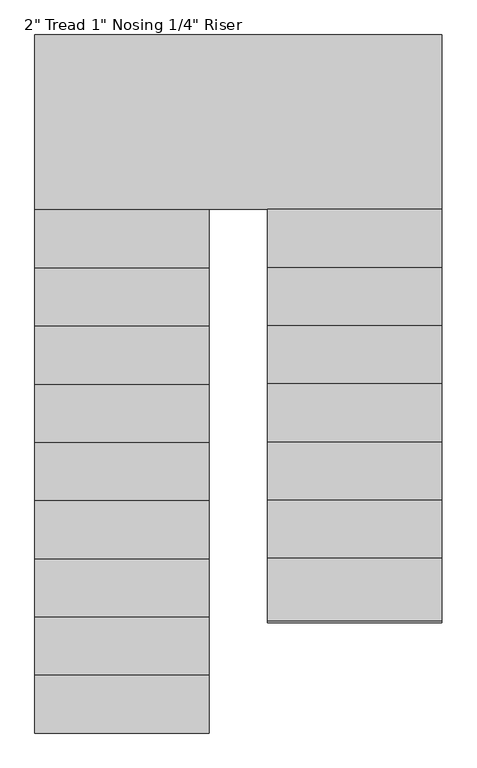
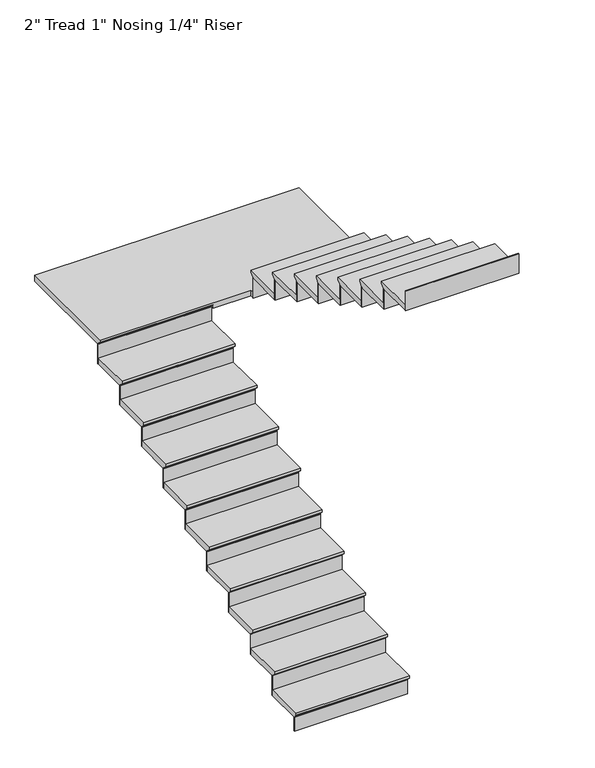
"""IFC4 building model written with IfcOpenShell, lengths in millimetres: stair flight geometry."""

from ifc_helpers import new_model, si_unit, origin, place, context, project, spatial, faceted_brep, source, transform, mapped, element, save


def stair_flight_2b6aeb10(model_context):
    return source(origin(), model_context, "Body", "Brep", [
        faceted_brep([(-77.7175798, -5516.2061634, 455.0833333), (-77.7175798, -5516.2061634, 474.1333333), (-992.1175798, -5516.2061634, 474.1333333), (-992.1175798, -5516.2061634, 455.0833333), (-77.7175798, -5490.8061634, 429.6833333), (-992.1175798, -5490.8061634, 429.6833333), (-77.7175798, -5186.0061634, 474.1333333), (-992.1175798, -5186.0061634, 474.1333333), (-992.1175798, -5490.8061634, 423.3333333), (-992.1175798, -5186.0061634, 423.3333333), (-77.7175798, -5186.0061634, 423.3333333), (-77.7175798, -5490.8061634, 423.3333333)], [[[0, 1, 2, 3]], [[4, 0, 3, 5]], [[2, 1, 6, 7]], [[8, 9, 10, 11]], [[2, 7, 9, 8, 5, 3]], [[8, 11, 4, 5]], [[6, 1, 0, 4, 11, 10]], [[7, 6, 10, 9]]]),
        faceted_brep([(-77.7175798, -5490.8061634, 423.3333333), (-77.7175798, -5490.8061634, 304.8), (-77.7175798, -5484.4561634, 304.8), (-77.7175798, -5484.4561634, 423.3333333), (-992.1175798, -5490.8061634, 423.3333333), (-992.1175798, -5484.4561634, 423.3333333), (-992.1175798, -5484.4561634, 304.8), (-992.1175798, -5490.8061634, 304.8)], [[[0, 1, 2, 3]], [[4, 5, 6, 7]], [[1, 0, 4, 7]], [[2, 1, 7, 6]], [[3, 2, 6, 5]], [[0, 3, 5, 4]]]),
        faceted_brep([(-77.7175798, -5186.0061634, 592.6666667), (-77.7175798, -5186.0061634, 423.3333333), (-77.7175798, -5179.6561634, 423.3333333), (-77.7175798, -5179.6561634, 592.6666667), (-992.1175798, -5186.0061634, 592.6666667), (-992.1175798, -5179.6561634, 592.6666667), (-992.1175798, -5179.6561634, 423.3333333), (-992.1175798, -5186.0061634, 423.3333333)], [[[0, 1, 2, 3]], [[4, 5, 6, 7]], [[1, 0, 4, 7]], [[2, 1, 7, 6]], [[3, 2, 6, 5]], [[0, 3, 5, 4]]]),
        faceted_brep([(-992.1175798, -5211.4061634, 643.4666667), (-77.7175798, -5211.4061634, 643.4666667), (-77.7175798, -4881.2061634, 643.4666667), (-992.1175798, -4881.2061634, 643.4666667), (-992.1175798, -5186.0061634, 592.6666667), (-992.1175798, -4881.2061634, 592.6666667), (-77.7175798, -4881.2061634, 592.6666667), (-77.7175798, -5186.0061634, 592.6666667), (-992.1175798, -5186.0061634, 599.0166667), (-992.1175798, -5211.4061634, 624.4166667), (-77.7175798, -5186.0061634, 599.0166667), (-77.7175798, -5211.4061634, 624.4166667)], [[[0, 1, 2, 3]], [[4, 5, 6, 7]], [[0, 3, 5, 4, 8, 9]], [[4, 7, 10, 8]], [[2, 1, 11, 10, 7, 6]], [[3, 2, 6, 5]], [[11, 1, 0, 9]], [[10, 11, 9, 8]]]),
        faceted_brep([(-77.7175798, -4881.2061634, 762.0), (-77.7175798, -4881.2061634, 592.6666667), (-77.7175798, -4874.8561634, 592.6666667), (-77.7175798, -4874.8561634, 762.0), (-992.1175798, -4881.2061634, 762.0), (-992.1175798, -4874.8561634, 762.0), (-992.1175798, -4874.8561634, 592.6666667), (-992.1175798, -4881.2061634, 592.6666667)], [[[0, 1, 2, 3]], [[4, 5, 6, 7]], [[1, 0, 4, 7]], [[2, 1, 7, 6]], [[3, 2, 6, 5]], [[0, 3, 5, 4]]]),
        faceted_brep([(-992.1175798, -4906.6061634, 812.8), (-77.7175798, -4906.6061634, 812.8), (-77.7175798, -4576.4061634, 812.8), (-992.1175798, -4576.4061634, 812.8), (-992.1175798, -4881.2061634, 762.0), (-992.1175798, -4576.4061634, 762.0), (-77.7175798, -4576.4061634, 762.0), (-77.7175798, -4881.2061634, 762.0), (-992.1175798, -4881.2061634, 768.35), (-992.1175798, -4906.6061634, 793.75), (-77.7175798, -4881.2061634, 768.35), (-77.7175798, -4906.6061634, 793.75)], [[[0, 1, 2, 3]], [[4, 5, 6, 7]], [[0, 3, 5, 4, 8, 9]], [[4, 7, 10, 8]], [[2, 1, 11, 10, 7, 6]], [[3, 2, 6, 5]], [[11, 1, 0, 9]], [[10, 11, 9, 8]]]),
        faceted_brep([(-77.7175798, -4576.4061634, 931.3333333), (-77.7175798, -4576.4061634, 762.0), (-77.7175798, -4570.0561634, 762.0), (-77.7175798, -4570.0561634, 931.3333333), (-992.1175798, -4576.4061634, 931.3333333), (-992.1175798, -4570.0561634, 931.3333333), (-992.1175798, -4570.0561634, 762.0), (-992.1175798, -4576.4061634, 762.0)], [[[0, 1, 2, 3]], [[4, 5, 6, 7]], [[1, 0, 4, 7]], [[2, 1, 7, 6]], [[3, 2, 6, 5]], [[0, 3, 5, 4]]]),
        faceted_brep([(-992.1175798, -4601.8061634, 982.1333333), (-77.7175798, -4601.8061634, 982.1333333), (-77.7175798, -4271.6061634, 982.1333333), (-992.1175798, -4271.6061634, 982.1333333), (-992.1175798, -4576.4061634, 931.3333333), (-992.1175798, -4271.6061634, 931.3333333), (-77.7175798, -4271.6061634, 931.3333333), (-77.7175798, -4576.4061634, 931.3333333), (-992.1175798, -4576.4061634, 937.6833333), (-992.1175798, -4601.8061634, 963.0833333), (-77.7175798, -4576.4061634, 937.6833333), (-77.7175798, -4601.8061634, 963.0833333)], [[[0, 1, 2, 3]], [[4, 5, 6, 7]], [[0, 3, 5, 4, 8, 9]], [[4, 7, 10, 8]], [[2, 1, 11, 10, 7, 6]], [[3, 2, 6, 5]], [[11, 1, 0, 9]], [[10, 11, 9, 8]]]),
        faceted_brep([(-77.7175798, -4271.6061634, 1100.6666667), (-77.7175798, -4271.6061634, 931.3333333), (-77.7175798, -4265.2561634, 931.3333333), (-77.7175798, -4265.2561634, 1100.6666667), (-992.1175798, -4271.6061634, 1100.6666667), (-992.1175798, -4265.2561634, 1100.6666667), (-992.1175798, -4265.2561634, 931.3333333), (-992.1175798, -4271.6061634, 931.3333333)], [[[0, 1, 2, 3]], [[4, 5, 6, 7]], [[1, 0, 4, 7]], [[2, 1, 7, 6]], [[3, 2, 6, 5]], [[0, 3, 5, 4]]]),
        faceted_brep([(-992.1175798, -4297.0061634, 1151.4666667), (-77.7175798, -4297.0061634, 1151.4666667), (-77.7175798, -3966.8061634, 1151.4666667), (-992.1175798, -3966.8061634, 1151.4666667), (-992.1175798, -4271.6061634, 1100.6666667), (-992.1175798, -3966.8061634, 1100.6666667), (-77.7175798, -3966.8061634, 1100.6666667), (-77.7175798, -4271.6061634, 1100.6666667), (-992.1175798, -4271.6061634, 1107.0166667), (-992.1175798, -4297.0061634, 1132.4166667), (-77.7175798, -4271.6061634, 1107.0166667), (-77.7175798, -4297.0061634, 1132.4166667)], [[[0, 1, 2, 3]], [[4, 5, 6, 7]], [[0, 3, 5, 4, 8, 9]], [[4, 7, 10, 8]], [[2, 1, 11, 10, 7, 6]], [[3, 2, 6, 5]], [[11, 1, 0, 9]], [[10, 11, 9, 8]]]),
        faceted_brep([(-77.7175798, -3966.8061634, 1270.0), (-77.7175798, -3966.8061634, 1100.6666667), (-77.7175798, -3960.4561634, 1100.6666667), (-77.7175798, -3960.4561634, 1270.0), (-992.1175798, -3966.8061634, 1270.0), (-992.1175798, -3960.4561634, 1270.0), (-992.1175798, -3960.4561634, 1100.6666667), (-992.1175798, -3966.8061634, 1100.6666667)], [[[0, 1, 2, 3]], [[4, 5, 6, 7]], [[1, 0, 4, 7]], [[2, 1, 7, 6]], [[3, 2, 6, 5]], [[0, 3, 5, 4]]]),
        faceted_brep([(-992.1175798, -3992.2061634, 1320.8), (-77.7175798, -3992.2061634, 1320.8), (-77.7175798, -3662.0061634, 1320.8), (-992.1175798, -3662.0061634, 1320.8), (-992.1175798, -3966.8061634, 1270.0), (-992.1175798, -3662.0061634, 1270.0), (-77.7175798, -3662.0061634, 1270.0), (-77.7175798, -3966.8061634, 1270.0), (-992.1175798, -3966.8061634, 1276.35), (-992.1175798, -3992.2061634, 1301.75), (-77.7175798, -3966.8061634, 1276.35), (-77.7175798, -3992.2061634, 1301.75)], [[[0, 1, 2, 3]], [[4, 5, 6, 7]], [[0, 3, 5, 4, 8, 9]], [[4, 7, 10, 8]], [[2, 1, 11, 10, 7, 6]], [[3, 2, 6, 5]], [[11, 1, 0, 9]], [[10, 11, 9, 8]]]),
        faceted_brep([(-77.7175798, -3662.0061634, 1439.3333333), (-77.7175798, -3662.0061634, 1270.0), (-77.7175798, -3655.6561634, 1270.0), (-77.7175798, -3655.6561634, 1439.3333333), (-992.1175798, -3662.0061634, 1439.3333333), (-992.1175798, -3655.6561634, 1439.3333333), (-992.1175798, -3655.6561634, 1270.0), (-992.1175798, -3662.0061634, 1270.0)], [[[0, 1, 2, 3]], [[4, 5, 6, 7]], [[1, 0, 4, 7]], [[2, 1, 7, 6]], [[3, 2, 6, 5]], [[0, 3, 5, 4]]]),
        faceted_brep([(-992.1175798, -3687.4061634, 1490.1333333), (-77.7175798, -3687.4061634, 1490.1333333), (-77.7175798, -3357.2061634, 1490.1333333), (-992.1175798, -3357.2061634, 1490.1333333), (-992.1175798, -3662.0061634, 1439.3333333), (-992.1175798, -3357.2061634, 1439.3333333), (-77.7175798, -3357.2061634, 1439.3333333), (-77.7175798, -3662.0061634, 1439.3333333), (-992.1175798, -3662.0061634, 1445.6833333), (-992.1175798, -3687.4061634, 1471.0833333), (-77.7175798, -3662.0061634, 1445.6833333), (-77.7175798, -3687.4061634, 1471.0833333)], [[[0, 1, 2, 3]], [[4, 5, 6, 7]], [[0, 3, 5, 4, 8, 9]], [[4, 7, 10, 8]], [[2, 1, 11, 10, 7, 6]], [[3, 2, 6, 5]], [[11, 1, 0, 9]], [[10, 11, 9, 8]]]),
        faceted_brep([(-77.7175798, -3357.2061634, 1608.6666667), (-77.7175798, -3357.2061634, 1439.3333333), (-77.7175798, -3350.8561634, 1439.3333333), (-77.7175798, -3350.8561634, 1608.6666667), (-992.1175798, -3357.2061634, 1608.6666667), (-992.1175798, -3350.8561634, 1608.6666667), (-992.1175798, -3350.8561634, 1439.3333333), (-992.1175798, -3357.2061634, 1439.3333333)], [[[0, 1, 2, 3]], [[4, 5, 6, 7]], [[1, 0, 4, 7]], [[2, 1, 7, 6]], [[3, 2, 6, 5]], [[0, 3, 5, 4]]]),
        faceted_brep([(-992.1175798, -3382.6061634, 1659.4666667), (-77.7175798, -3382.6061634, 1659.4666667), (-77.7175798, -3052.4061634, 1659.4666667), (-992.1175798, -3052.4061634, 1659.4666667), (-992.1175798, -3357.2061634, 1608.6666667), (-992.1175798, -3052.4061634, 1608.6666667), (-77.7175798, -3052.4061634, 1608.6666667), (-77.7175798, -3357.2061634, 1608.6666667), (-992.1175798, -3357.2061634, 1615.0166667), (-992.1175798, -3382.6061634, 1640.4166667), (-77.7175798, -3357.2061634, 1615.0166667), (-77.7175798, -3382.6061634, 1640.4166667)], [[[0, 1, 2, 3]], [[4, 5, 6, 7]], [[0, 3, 5, 4, 8, 9]], [[4, 7, 10, 8]], [[2, 1, 11, 10, 7, 6]], [[3, 2, 6, 5]], [[11, 1, 0, 9]], [[10, 11, 9, 8]]]),
        faceted_brep([(-77.7175798, -3052.4061634, 1778.0), (-77.7175798, -3052.4061634, 1608.6666667), (-77.7175798, -3046.0561634, 1608.6666667), (-77.7175798, -3046.0561634, 1778.0), (-992.1175798, -3052.4061634, 1778.0), (-992.1175798, -3046.0561634, 1778.0), (-992.1175798, -3046.0561634, 1608.6666667), (-992.1175798, -3052.4061634, 1608.6666667)], [[[0, 1, 2, 3]], [[4, 5, 6, 7]], [[1, 0, 4, 7]], [[2, 1, 7, 6]], [[3, 2, 6, 5]], [[0, 3, 5, 4]]]),
        faceted_brep([(-992.1175798, -3077.8061634, 1828.8), (-77.7175798, -3077.8061634, 1828.8), (-77.7175798, -2747.6061634, 1828.8), (-992.1175798, -2747.6061634, 1828.8), (-992.1175798, -3052.4061634, 1778.0), (-992.1175798, -2747.6061634, 1778.0), (-77.7175798, -2747.6061634, 1778.0), (-77.7175798, -3052.4061634, 1778.0), (-992.1175798, -3052.4061634, 1784.35), (-992.1175798, -3077.8061634, 1809.75), (-77.7175798, -3052.4061634, 1784.35), (-77.7175798, -3077.8061634, 1809.75)], [[[0, 1, 2, 3]], [[4, 5, 6, 7]], [[0, 3, 5, 4, 8, 9]], [[4, 7, 10, 8]], [[2, 1, 11, 10, 7, 6]], [[3, 2, 6, 5]], [[11, 1, 0, 9]], [[10, 11, 9, 8]]]),
        faceted_brep([(-77.7175798, -2747.6061634, 1947.3333333), (-77.7175798, -2747.6061634, 1778.0), (-77.7175798, -2741.2561634, 1778.0), (-77.7175798, -2741.2561634, 1947.3333333), (-992.1175798, -2747.6061634, 1947.3333333), (-992.1175798, -2741.2561634, 1947.3333333), (-992.1175798, -2741.2561634, 1778.0), (-992.1175798, -2747.6061634, 1778.0)], [[[0, 1, 2, 3]], [[4, 5, 6, 7]], [[1, 0, 4, 7]], [[2, 1, 7, 6]], [[3, 2, 6, 5]], [[0, 3, 5, 4]]]),
        faceted_brep([(1141.4824202, -2798.4061634, 1998.1333333), (1141.4824202, -1858.6061634, 1998.1333333), (-992.1175798, -1858.6061634, 1998.1333333), (-992.1175798, -2773.0061634, 1998.1333333), (227.0824202, -2773.0061634, 1998.1333333), (227.0824202, -2798.4061634, 1998.1333333), (1141.4824202, -1858.6061634, 1947.3333333), (1141.4824202, -2798.4061634, 1947.3333333), (227.0824202, -2798.4061634, 1947.3333333), (227.0824202, -2773.0061634, 1947.3333333), (-77.7175798, -2773.0061634, 1947.3333333), (-77.7175798, -2747.6061634, 1947.3333333), (-992.1175798, -2747.6061634, 1947.3333333), (-992.1175798, -1858.6061634, 1947.3333333), (-992.1175798, -2747.6061634, 1953.6833333), (-992.1175798, -2773.0061634, 1979.0833333), (-77.7175798, -2747.6061634, 1953.6833333), (-77.7175798, -2773.0061634, 1979.0833333)], [[[0, 1, 2, 3, 4, 5]], [[6, 7, 8, 9, 10, 11, 12, 13]], [[1, 0, 7, 6]], [[2, 1, 6, 13]], [[3, 2, 13, 12, 14, 15]], [[12, 11, 16, 14]], [[11, 10, 17, 16]], [[4, 3, 15, 17, 10, 9]], [[5, 4, 9, 8]], [[0, 5, 8, 7]], [[15, 14, 16, 17]]]),
        faceted_brep([(227.0824202, -2798.4061634, 2116.6666667), (227.0824202, -2798.4061634, 1947.3333333), (227.0824202, -2804.7561634, 1947.3333333), (227.0824202, -2804.7561634, 2116.6666667), (1141.4824202, -2798.4061634, 2116.6666667), (1141.4824202, -2804.7561634, 2116.6666667), (1141.4824202, -2804.7561634, 1947.3333333), (1141.4824202, -2798.4061634, 1947.3333333)], [[[0, 1, 2, 3]], [[4, 5, 6, 7]], [[1, 0, 4, 7]], [[2, 1, 7, 6]], [[3, 2, 6, 5]], [[0, 3, 5, 4]]]),
        faceted_brep([(1141.4824202, -2773.0061634, 2167.4666667), (227.0824202, -2773.0061634, 2167.4666667), (227.0824202, -3103.2061634, 2167.4666667), (1141.4824202, -3103.2061634, 2167.4666667), (1141.4824202, -2798.4061634, 2116.6666667), (1141.4824202, -3103.2061634, 2116.6666667), (227.0824202, -3103.2061634, 2116.6666667), (227.0824202, -2798.4061634, 2116.6666667), (1141.4824202, -2798.4061634, 2123.0166667), (1141.4824202, -2773.0061634, 2148.4166667), (227.0824202, -2798.4061634, 2123.0166667), (227.0824202, -2773.0061634, 2148.4166667)], [[[0, 1, 2, 3]], [[4, 5, 6, 7]], [[0, 3, 5, 4, 8, 9]], [[4, 7, 10, 8]], [[2, 1, 11, 10, 7, 6]], [[3, 2, 6, 5]], [[11, 1, 0, 9]], [[10, 11, 9, 8]]]),
        faceted_brep([(227.0824202, -3103.2061634, 2286.0), (227.0824202, -3103.2061634, 2116.6666667), (227.0824202, -3109.5561634, 2116.6666667), (227.0824202, -3109.5561634, 2286.0), (1141.4824202, -3103.2061634, 2286.0), (1141.4824202, -3109.5561634, 2286.0), (1141.4824202, -3109.5561634, 2116.6666667), (1141.4824202, -3103.2061634, 2116.6666667)], [[[0, 1, 2, 3]], [[4, 5, 6, 7]], [[1, 0, 4, 7]], [[2, 1, 7, 6]], [[3, 2, 6, 5]], [[0, 3, 5, 4]]]),
        faceted_brep([(1141.4824202, -3077.8061634, 2336.8), (227.0824202, -3077.8061634, 2336.8), (227.0824202, -3408.0061634, 2336.8), (1141.4824202, -3408.0061634, 2336.8), (1141.4824202, -3103.2061634, 2286.0), (1141.4824202, -3408.0061634, 2286.0), (227.0824202, -3408.0061634, 2286.0), (227.0824202, -3103.2061634, 2286.0), (1141.4824202, -3103.2061634, 2292.35), (1141.4824202, -3077.8061634, 2317.75), (227.0824202, -3103.2061634, 2292.35), (227.0824202, -3077.8061634, 2317.75)], [[[0, 1, 2, 3]], [[4, 5, 6, 7]], [[0, 3, 5, 4, 8, 9]], [[4, 7, 10, 8]], [[2, 1, 11, 10, 7, 6]], [[3, 2, 6, 5]], [[11, 1, 0, 9]], [[10, 11, 9, 8]]]),
        faceted_brep([(227.0824202, -3408.0061634, 2455.3333333), (227.0824202, -3408.0061634, 2286.0), (227.0824202, -3414.3561634, 2286.0), (227.0824202, -3414.3561634, 2455.3333333), (1141.4824202, -3408.0061634, 2455.3333333), (1141.4824202, -3414.3561634, 2455.3333333), (1141.4824202, -3414.3561634, 2286.0), (1141.4824202, -3408.0061634, 2286.0)], [[[0, 1, 2, 3]], [[4, 5, 6, 7]], [[1, 0, 4, 7]], [[2, 1, 7, 6]], [[3, 2, 6, 5]], [[0, 3, 5, 4]]]),
        faceted_brep([(1141.4824202, -3382.6061634, 2506.1333333), (227.0824202, -3382.6061634, 2506.1333333), (227.0824202, -3712.8061634, 2506.1333333), (1141.4824202, -3712.8061634, 2506.1333333), (1141.4824202, -3408.0061634, 2455.3333333), (1141.4824202, -3712.8061634, 2455.3333333), (227.0824202, -3712.8061634, 2455.3333333), (227.0824202, -3408.0061634, 2455.3333333), (1141.4824202, -3408.0061634, 2461.6833333), (1141.4824202, -3382.6061634, 2487.0833333), (227.0824202, -3408.0061634, 2461.6833333), (227.0824202, -3382.6061634, 2487.0833333)], [[[0, 1, 2, 3]], [[4, 5, 6, 7]], [[0, 3, 5, 4, 8, 9]], [[4, 7, 10, 8]], [[2, 1, 11, 10, 7, 6]], [[3, 2, 6, 5]], [[11, 1, 0, 9]], [[10, 11, 9, 8]]]),
        faceted_brep([(227.0824202, -3712.8061634, 2624.6666667), (227.0824202, -3712.8061634, 2455.3333333), (227.0824202, -3719.1561634, 2455.3333333), (227.0824202, -3719.1561634, 2624.6666667), (1141.4824202, -3712.8061634, 2624.6666667), (1141.4824202, -3719.1561634, 2624.6666667), (1141.4824202, -3719.1561634, 2455.3333333), (1141.4824202, -3712.8061634, 2455.3333333)], [[[0, 1, 2, 3]], [[4, 5, 6, 7]], [[1, 0, 4, 7]], [[2, 1, 7, 6]], [[3, 2, 6, 5]], [[0, 3, 5, 4]]]),
        faceted_brep([(1141.4824202, -3687.4061634, 2675.4666667), (227.0824202, -3687.4061634, 2675.4666667), (227.0824202, -4017.6061634, 2675.4666667), (1141.4824202, -4017.6061634, 2675.4666667), (1141.4824202, -3712.8061634, 2624.6666667), (1141.4824202, -4017.6061634, 2624.6666667), (227.0824202, -4017.6061634, 2624.6666667), (227.0824202, -3712.8061634, 2624.6666667), (1141.4824202, -3712.8061634, 2631.0166667), (1141.4824202, -3687.4061634, 2656.4166667), (227.0824202, -3712.8061634, 2631.0166667), (227.0824202, -3687.4061634, 2656.4166667)], [[[0, 1, 2, 3]], [[4, 5, 6, 7]], [[0, 3, 5, 4, 8, 9]], [[4, 7, 10, 8]], [[2, 1, 11, 10, 7, 6]], [[3, 2, 6, 5]], [[11, 1, 0, 9]], [[10, 11, 9, 8]]]),
        faceted_brep([(227.0824202, -4017.6061634, 2794.0), (227.0824202, -4017.6061634, 2624.6666667), (227.0824202, -4023.9561634, 2624.6666667), (227.0824202, -4023.9561634, 2794.0), (1141.4824202, -4017.6061634, 2794.0), (1141.4824202, -4023.9561634, 2794.0), (1141.4824202, -4023.9561634, 2624.6666667), (1141.4824202, -4017.6061634, 2624.6666667)], [[[0, 1, 2, 3]], [[4, 5, 6, 7]], [[1, 0, 4, 7]], [[2, 1, 7, 6]], [[3, 2, 6, 5]], [[0, 3, 5, 4]]]),
        faceted_brep([(1141.4824202, -3992.2061634, 2844.8), (227.0824202, -3992.2061634, 2844.8), (227.0824202, -4322.4061634, 2844.8), (1141.4824202, -4322.4061634, 2844.8), (1141.4824202, -4017.6061634, 2794.0), (1141.4824202, -4322.4061634, 2794.0), (227.0824202, -4322.4061634, 2794.0), (227.0824202, -4017.6061634, 2794.0), (1141.4824202, -4017.6061634, 2800.35), (1141.4824202, -3992.2061634, 2825.75), (227.0824202, -4017.6061634, 2800.35), (227.0824202, -3992.2061634, 2825.75)], [[[0, 1, 2, 3]], [[4, 5, 6, 7]], [[0, 3, 5, 4, 8, 9]], [[4, 7, 10, 8]], [[2, 1, 11, 10, 7, 6]], [[3, 2, 6, 5]], [[11, 1, 0, 9]], [[10, 11, 9, 8]]]),
        faceted_brep([(227.0824202, -4322.4061634, 2963.3333333), (227.0824202, -4322.4061634, 2794.0), (227.0824202, -4328.7561634, 2794.0), (227.0824202, -4328.7561634, 2963.3333333), (1141.4824202, -4322.4061634, 2963.3333333), (1141.4824202, -4328.7561634, 2963.3333333), (1141.4824202, -4328.7561634, 2794.0), (1141.4824202, -4322.4061634, 2794.0)], [[[0, 1, 2, 3]], [[4, 5, 6, 7]], [[1, 0, 4, 7]], [[2, 1, 7, 6]], [[3, 2, 6, 5]], [[0, 3, 5, 4]]]),
        faceted_brep([(1141.4824202, -4297.0061634, 3014.1333333), (227.0824202, -4297.0061634, 3014.1333333), (227.0824202, -4627.2061634, 3014.1333333), (1141.4824202, -4627.2061634, 3014.1333333), (1141.4824202, -4322.4061634, 2963.3333333), (1141.4824202, -4627.2061634, 2963.3333333), (227.0824202, -4627.2061634, 2963.3333333), (227.0824202, -4322.4061634, 2963.3333333), (1141.4824202, -4322.4061634, 2969.6833333), (1141.4824202, -4297.0061634, 2995.0833333), (227.0824202, -4322.4061634, 2969.6833333), (227.0824202, -4297.0061634, 2995.0833333)], [[[0, 1, 2, 3]], [[4, 5, 6, 7]], [[0, 3, 5, 4, 8, 9]], [[4, 7, 10, 8]], [[2, 1, 11, 10, 7, 6]], [[3, 2, 6, 5]], [[11, 1, 0, 9]], [[10, 11, 9, 8]]]),
        faceted_brep([(227.0824202, -4627.2061634, 3132.6666667), (227.0824202, -4627.2061634, 2963.3333333), (227.0824202, -4633.5561634, 2963.3333333), (227.0824202, -4633.5561634, 3132.6666667), (1141.4824202, -4627.2061634, 3132.6666667), (1141.4824202, -4633.5561634, 3132.6666667), (1141.4824202, -4633.5561634, 2963.3333333), (1141.4824202, -4627.2061634, 2963.3333333)], [[[0, 1, 2, 3]], [[4, 5, 6, 7]], [[1, 0, 4, 7]], [[2, 1, 7, 6]], [[3, 2, 6, 5]], [[0, 3, 5, 4]]]),
        faceted_brep([(227.0824202, -4932.0061634, 3302.0), (227.0824202, -4932.0061634, 3132.6666667), (227.0824202, -4938.3561634, 3132.6666667), (227.0824202, -4938.3561634, 3302.0), (1141.4824202, -4932.0061634, 3302.0), (1141.4824202, -4938.3561634, 3302.0), (1141.4824202, -4938.3561634, 3132.6666667), (1141.4824202, -4932.0061634, 3132.6666667)], [[[0, 1, 2, 3]], [[4, 5, 6, 7]], [[1, 0, 4, 7]], [[2, 1, 7, 6]], [[3, 2, 6, 5]], [[0, 3, 5, 4]]]),
        faceted_brep([(1141.4824202, -4601.8061634, 3183.4666667), (227.0824202, -4601.8061634, 3183.4666667), (227.0824202, -4932.0061634, 3183.4666667), (1141.4824202, -4932.0061634, 3183.4666667), (1141.4824202, -4627.2061634, 3132.6666667), (1141.4824202, -4932.0061634, 3132.6666667), (227.0824202, -4932.0061634, 3132.6666667), (227.0824202, -4627.2061634, 3132.6666667), (1141.4824202, -4627.2061634, 3139.0166667), (1141.4824202, -4601.8061634, 3164.4166667), (227.0824202, -4627.2061634, 3139.0166667), (227.0824202, -4601.8061634, 3164.4166667)], [[[0, 1, 2, 3]], [[4, 5, 6, 7]], [[0, 3, 5, 4, 8, 9]], [[4, 7, 10, 8]], [[2, 1, 11, 10, 7, 6]], [[3, 2, 6, 5]], [[11, 1, 0, 9]], [[10, 11, 9, 8]]]),
    ])


if __name__ == "__main__":
    model = new_model("IFC4")
    model_context = context("Model", 3, world=origin())
    ifc_project = project(units=[si_unit("LENGTHUNIT", "METRE", prefix="MILLI")], contexts=[model_context])
    site = spatial("IfcSite", under=ifc_project)
    building = spatial("IfcBuilding", under=site)
    placement = place(None, origin())
    stair_flight_shape = stair_flight_2b6aeb10(model_context)
    element("IfcStairFlight", 1, ObjectType="2\" Tread 1\" Nosing 1/4\" Riser", at=placement, inside=building, context=model_context, shape_type="MappedRepresentation", body=[
        mapped(stair_flight_shape, transform((0.0, 0.0, 0.0), x_axis=(1.0, 0.0, 0.0), y_axis=(0.0, 1.0, 0.0), z_axis=(0.0, 0.0, 1.0))),
    ])
    save(model, "model.ifc")

# Revit data of these elements
# Element 1 (IfcStairFlight, "2\" Tread 1\" Nosing 1/4\" Riser")
#   Materials on its faces: "FL_MARBLE WHITE"
# Materials
#   "FL_MARBLE WHITE": class "Generic", colour RGB 120 120 120, transparency 0, Cost = 0
